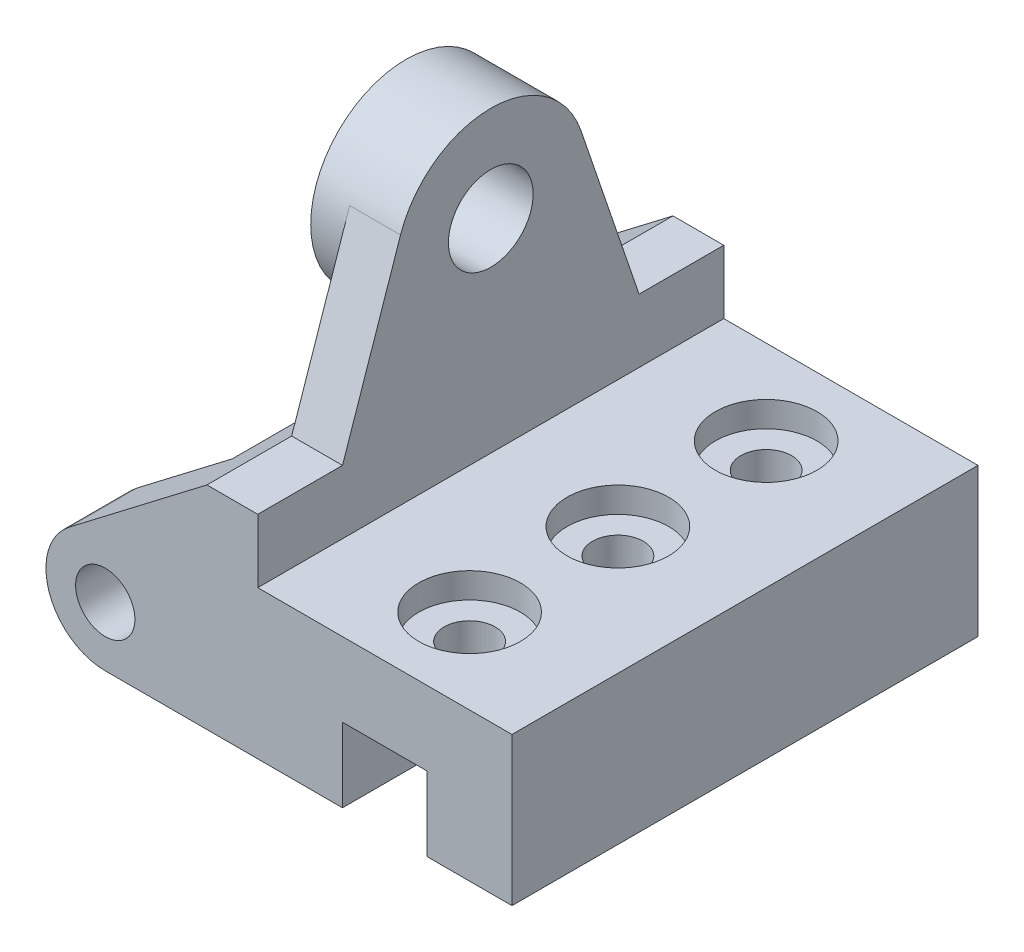
ISO-10303-21;
HEADER;
FILE_DESCRIPTION(('STEP AP214'),'2;1');
FILE_NAME('part.step','',(''),(''),'','','');
FILE_SCHEMA(('AUTOMOTIVE_DESIGN { 1 0 10303 214 1 1 1 1 }'));
ENDSEC;
DATA;
#1=APPLICATION_CONTEXT('core data for automotive mechanical design processes');
#2=APPLICATION_PROTOCOL_DEFINITION('international standard','automotive_design',2000,#1);
#3=PRODUCT_CONTEXT('',#1,'mechanical');
#4=PRODUCT('Part','Part','',(#3));
#5=PRODUCT_RELATED_PRODUCT_CATEGORY('part','',(#4));
#6=PRODUCT_DEFINITION_FORMATION('','',#4);
#7=PRODUCT_DEFINITION_CONTEXT('part definition',#1,'design');
#8=PRODUCT_DEFINITION('design','',#6,#7);
#9=PRODUCT_DEFINITION_SHAPE('','',#8);
#10=(LENGTH_UNIT() NAMED_UNIT(*) SI_UNIT(.MILLI.,.METRE.));
#11=(NAMED_UNIT(*) PLANE_ANGLE_UNIT() SI_UNIT($,.RADIAN.));
#12=(NAMED_UNIT(*) SI_UNIT($,.STERADIAN.) SOLID_ANGLE_UNIT());
#13=UNCERTAINTY_MEASURE_WITH_UNIT(LENGTH_MEASURE(1.E-05),#10,'distance_accuracy_value','');
#14=(GEOMETRIC_REPRESENTATION_CONTEXT(3) GLOBAL_UNCERTAINTY_ASSIGNED_CONTEXT((#13)) GLOBAL_UNIT_ASSIGNED_CONTEXT((#10,
#11,#12)) REPRESENTATION_CONTEXT('',''));
#15=CARTESIAN_POINT('',(0.,0.,0.));
#16=DIRECTION('',(0.,0.,1.));
#17=DIRECTION('',(1.,0.,0.));
#18=AXIS2_PLACEMENT_3D('',#15,#16,#17);
#19=CARTESIAN_POINT('',(24.,69.,0.));
#20=DIRECTION('',(1.,0.,0.));
#21=DIRECTION('',(0.,0.,-1.));
#22=AXIS2_PLACEMENT_3D('',#19,#20,#21);
#23=PLANE('',#22);
#24=CARTESIAN_POINT('',(24.,69.,0.));
#25=DIRECTION('',(-1.,0.,0.));
#26=DIRECTION('',(0.,0.,1.));
#27=AXIS2_PLACEMENT_3D('',#24,#25,#26);
#28=CIRCLE('',#27,22.5);
#29=CARTESIAN_POINT('',(24.,76.2499542674237,-21.2999568807138));
#30=VERTEX_POINT('',#29);
#31=CARTESIAN_POINT('',(24.,76.2499542674237,21.2999568807138));
#32=VERTEX_POINT('',#31);
#33=EDGE_CURVE('E176',#30,#32,#28,.T.);
#34=ORIENTED_EDGE('',*,*,#33,.F.);
#35=DIRECTION('',(0.,0.946664750253944,0.322220189663274));
#36=VECTOR('',#35,1.);
#37=CARTESIAN_POINT('',(24.,36.,-35.));
#38=LINE('',#37,#36);
#39=CARTESIAN_POINT('',(24.,36.,-35.));
#40=VERTEX_POINT('',#39);
#41=EDGE_CURVE('E189',#40,#30,#38,.T.);
#42=ORIENTED_EDGE('',*,*,#41,.F.);
#43=DIRECTION('',(0.,0.,-1.));
#44=VECTOR('',#43,1.);
#45=CARTESIAN_POINT('',(24.,36.,-35.));
#46=LINE('',#45,#44);
#47=CARTESIAN_POINT('',(24.,36.,35.));
#48=VERTEX_POINT('',#47);
#49=EDGE_CURVE('E181',#48,#40,#46,.T.);
#50=ORIENTED_EDGE('',*,*,#49,.F.);
#51=DIRECTION('',(0.,-0.946664750253944,0.322220189663275));
#52=VECTOR('',#51,1.);
#53=CARTESIAN_POINT('',(24.,76.2499542674237,21.2999568807137));
#54=LINE('',#53,#52);
#55=EDGE_CURVE('E178',#32,#48,#54,.T.);
#56=ORIENTED_EDGE('',*,*,#55,.F.);
#57=EDGE_LOOP('',(#34,#42,#50,#56));
#58=FACE_BOUND('',#57,.T.);
#59=ADVANCED_FACE('F43',(#58),#23,.F.);
#60=CARTESIAN_POINT('',(36.,36.,-55.));
#61=DIRECTION('',(0.,1.,0.));
#62=DIRECTION('',(-1.,0.,0.));
#63=AXIS2_PLACEMENT_3D('',#60,#61,#62);
#64=PLANE('',#63);
#65=DIRECTION('',(0.,0.,1.));
#66=VECTOR('',#65,1.);
#67=CARTESIAN_POINT('',(24.,36.,-55.));
#68=LINE('',#67,#66);
#69=CARTESIAN_POINT('',(24.,36.,-55.));
#70=VERTEX_POINT('',#69);
#71=EDGE_CURVE('E317',#70,#40,#68,.T.);
#72=ORIENTED_EDGE('',*,*,#71,.T.);
#73=DIRECTION('',(1.,0.,0.));
#74=VECTOR('',#73,1.);
#75=CARTESIAN_POINT('',(24.,36.,-35.));
#76=LINE('',#75,#74);
#77=CARTESIAN_POINT('',(36.,36.,-35.));
#78=VERTEX_POINT('',#77);
#79=EDGE_CURVE('E188',#40,#78,#76,.T.);
#80=ORIENTED_EDGE('',*,*,#79,.T.);
#81=DIRECTION('',(0.,0.,1.));
#82=VECTOR('',#81,1.);
#83=CARTESIAN_POINT('',(36.,36.,-55.));
#84=LINE('',#83,#82);
#85=CARTESIAN_POINT('',(36.,36.,-55.));
#86=VERTEX_POINT('',#85);
#87=EDGE_CURVE('E323',#86,#78,#84,.T.);
#88=ORIENTED_EDGE('',*,*,#87,.F.);
#89=DIRECTION('',(-1.,0.,0.));
#90=VECTOR('',#89,1.);
#91=CARTESIAN_POINT('',(36.,36.,-55.));
#92=LINE('',#91,#90);
#93=EDGE_CURVE('E283',#86,#70,#92,.T.);
#94=ORIENTED_EDGE('',*,*,#93,.T.);
#95=EDGE_LOOP('',(#72,#80,#88,#94));
#96=FACE_BOUND('',#95,.T.);
#97=ADVANCED_FACE('F438',(#96),#64,.T.);
#98=CARTESIAN_POINT('',(0.,0.,-55.));
#99=DIRECTION('',(0.,0.,1.));
#100=DIRECTION('',(1.,0.,0.));
#101=AXIS2_PLACEMENT_3D('',#98,#99,#100);
#102=CYLINDRICAL_SURFACE('',#101,14.);
#103=CARTESIAN_POINT('',(0.,0.,39.));
#104=DIRECTION('',(0.,0.,1.));
#105=DIRECTION('',(1.,0.,0.));
#106=AXIS2_PLACEMENT_3D('',#103,#104,#105);
#107=CIRCLE('',#106,14.);
#108=CARTESIAN_POINT('',(0.,-14.,39.));
#109=VERTEX_POINT('',#108);
#110=CARTESIAN_POINT('',(-8.50921228973418,11.1172526376006,39.));
#111=VERTEX_POINT('',#110);
#112=EDGE_CURVE('E244',#109,#111,#107,.F.);
#113=ORIENTED_EDGE('',*,*,#112,.F.);
#114=DIRECTION('',(0.,0.,1.));
#115=VECTOR('',#114,1.);
#116=CARTESIAN_POINT('',(0.,-14.,-55.));
#117=LINE('',#116,#115);
#118=CARTESIAN_POINT('',(0.,-14.,55.));
#119=VERTEX_POINT('',#118);
#120=EDGE_CURVE('E289',#109,#119,#117,.T.);
#121=ORIENTED_EDGE('',*,*,#120,.T.);
#122=CARTESIAN_POINT('',(0.,0.,55.));
#123=DIRECTION('',(0.,0.,1.));
#124=DIRECTION('',(1.,0.,0.));
#125=AXIS2_PLACEMENT_3D('',#122,#123,#124);
#126=CIRCLE('',#125,14.);
#127=CARTESIAN_POINT('',(-8.50921228973418,11.1172526376006,55.));
#128=VERTEX_POINT('',#127);
#129=EDGE_CURVE('E246',#128,#119,#126,.T.);
#130=ORIENTED_EDGE('',*,*,#129,.F.);
#131=DIRECTION('',(0.,0.,1.));
#132=VECTOR('',#131,1.);
#133=CARTESIAN_POINT('',(-8.50921228973418,11.1172526376006,-55.));
#134=LINE('',#133,#132);
#135=EDGE_CURVE('E55',#111,#128,#134,.T.);
#136=ORIENTED_EDGE('',*,*,#135,.F.);
#137=EDGE_LOOP('',(#113,#121,#130,#136));
#138=FACE_BOUND('',#137,.T.);
#139=ADVANCED_FACE('F453',(#138),#102,.T.);
#140=CARTESIAN_POINT('',(0.,0.,-55.));
#141=DIRECTION('',(0.,0.,1.));
#142=DIRECTION('',(1.,0.,0.));
#143=AXIS2_PLACEMENT_3D('',#140,#141,#142);
#144=CYLINDRICAL_SURFACE('',#143,7.);
#145=CARTESIAN_POINT('',(0.,0.,39.));
#146=DIRECTION('',(0.,0.,1.));
#147=DIRECTION('',(1.,0.,0.));
#148=AXIS2_PLACEMENT_3D('',#145,#146,#147);
#149=CIRCLE('',#148,7.);
#150=CARTESIAN_POINT('',(7.,0.,39.));
#151=VERTEX_POINT('',#150);
#152=EDGE_CURVE('E239',#151,#151,#149,.F.);
#153=ORIENTED_EDGE('',*,*,#152,.T.);
#154=EDGE_LOOP('',(#153));
#155=FACE_BOUND('',#154,.T.);
#156=CARTESIAN_POINT('',(0.,0.,55.));
#157=DIRECTION('',(0.,0.,1.));
#158=DIRECTION('',(1.,0.,0.));
#159=AXIS2_PLACEMENT_3D('',#156,#157,#158);
#160=CIRCLE('',#159,7.);
#161=CARTESIAN_POINT('',(7.,0.,55.));
#162=VERTEX_POINT('',#161);
#163=EDGE_CURVE('E248',#162,#162,#160,.T.);
#164=ORIENTED_EDGE('',*,*,#163,.T.);
#165=EDGE_LOOP('',(#164));
#166=FACE_BOUND('',#165,.T.);
#167=ADVANCED_FACE('F466',(#155,#166),#144,.F.);
#168=CARTESIAN_POINT('',(0.,0.,-39.));
#169=DIRECTION('',(0.,0.,-1.));
#170=DIRECTION('',(-1.,0.,0.));
#171=AXIS2_PLACEMENT_3D('',#168,#169,#170);
#172=CIRCLE('',#171,14.);
#173=CARTESIAN_POINT('',(-8.50921228973418,11.1172526376006,-39.));
#174=VERTEX_POINT('',#173);
#175=CARTESIAN_POINT('',(0.,-14.,-39.));
#176=VERTEX_POINT('',#175);
#177=EDGE_CURVE('E67',#174,#176,#172,.F.);
#178=ORIENTED_EDGE('',*,*,#177,.F.);
#179=CARTESIAN_POINT('',(-8.50921228973418,11.1172526376006,-55.));
#180=VERTEX_POINT('',#179);
#181=EDGE_CURVE('E11',#180,#174,#134,.T.);
#182=ORIENTED_EDGE('',*,*,#181,.F.);
#183=CARTESIAN_POINT('',(0.,0.,-55.));
#184=DIRECTION('',(0.,0.,1.));
#185=DIRECTION('',(1.,0.,0.));
#186=AXIS2_PLACEMENT_3D('',#183,#184,#185);
#187=CIRCLE('',#186,14.);
#188=CARTESIAN_POINT('',(0.,-14.,-55.));
#189=VERTEX_POINT('',#188);
#190=EDGE_CURVE('E251',#180,#189,#187,.T.);
#191=ORIENTED_EDGE('',*,*,#190,.T.);
#192=EDGE_CURVE('E343',#189,#176,#117,.T.);
#193=ORIENTED_EDGE('',*,*,#192,.T.);
#194=EDGE_LOOP('',(#178,#182,#191,#193));
#195=FACE_BOUND('',#194,.T.);
#196=ADVANCED_FACE('F44',(#195),#102,.T.);
#197=CARTESIAN_POINT('',(24.,36.,-55.));
#198=DIRECTION('',(-0.607800877838156,0.794089474114326,0.));
#199=DIRECTION('',(-0.794089474114326,-0.607800877838156,0.));
#200=AXIS2_PLACEMENT_3D('',#197,#198,#199);
#201=PLANE('',#200);
#202=DIRECTION('',(0.794089474114326,0.607800877838156,0.));
#203=VECTOR('',#202,1.);
#204=CARTESIAN_POINT('',(24.,36.,39.));
#205=LINE('',#204,#203);
#206=CARTESIAN_POINT('',(14.,28.3459396245485,39.));
#207=VERTEX_POINT('',#206);
#208=EDGE_CURVE('E238',#111,#207,#205,.T.);
#209=ORIENTED_EDGE('',*,*,#208,.F.);
#210=ORIENTED_EDGE('',*,*,#135,.T.);
#211=DIRECTION('',(-0.794089474114326,-0.607800877838156,0.));
#212=VECTOR('',#211,1.);
#213=CARTESIAN_POINT('',(24.,36.,55.));
#214=LINE('',#213,#212);
#215=CARTESIAN_POINT('',(24.,36.,55.));
#216=VERTEX_POINT('',#215);
#217=EDGE_CURVE('E260',#216,#128,#214,.T.);
#218=ORIENTED_EDGE('',*,*,#217,.F.);
#219=EDGE_CURVE('E325',#48,#216,#68,.T.);
#220=ORIENTED_EDGE('',*,*,#219,.F.);
#221=ORIENTED_EDGE('',*,*,#49,.T.);
#222=ORIENTED_EDGE('',*,*,#71,.F.);
#223=DIRECTION('',(-0.794089474114326,-0.607800877838156,0.));
#224=VECTOR('',#223,1.);
#225=CARTESIAN_POINT('',(24.,36.,-55.));
#226=LINE('',#225,#224);
#227=EDGE_CURVE('E285',#70,#180,#226,.T.);
#228=ORIENTED_EDGE('',*,*,#227,.T.);
#229=ORIENTED_EDGE('',*,*,#181,.T.);
#230=DIRECTION('',(-0.794089474114326,-0.607800877838156,0.));
#231=VECTOR('',#230,1.);
#232=CARTESIAN_POINT('',(24.,36.,-39.));
#233=LINE('',#232,#231);
#234=CARTESIAN_POINT('',(14.,28.3459396245485,-39.));
#235=VERTEX_POINT('',#234);
#236=EDGE_CURVE('E237',#235,#174,#233,.T.);
#237=ORIENTED_EDGE('',*,*,#236,.F.);
#238=DIRECTION('',(0.,0.,-1.));
#239=VECTOR('',#238,1.);
#240=CARTESIAN_POINT('',(14.,28.3459396245485,-55.));
#241=LINE('',#240,#239);
#242=EDGE_CURVE('E245',#207,#235,#241,.T.);
#243=ORIENTED_EDGE('',*,*,#242,.F.);
#244=EDGE_LOOP('',(#209,#210,#218,#220,#221,#222,#228,#229,#237,#243));
#245=FACE_BOUND('',#244,.T.);
#246=ADVANCED_FACE('F434',(#245),#201,.T.);
#247=DIRECTION('',(1.,0.,0.));
#248=VECTOR('',#247,1.);
#249=CARTESIAN_POINT('',(24.,36.,35.));
#250=LINE('',#249,#248);
#251=CARTESIAN_POINT('',(36.,36.,35.));
#252=VERTEX_POINT('',#251);
#253=EDGE_CURVE('E197',#48,#252,#250,.T.);
#254=ORIENTED_EDGE('',*,*,#253,.F.);
#255=ORIENTED_EDGE('',*,*,#219,.T.);
#256=DIRECTION('',(-1.,0.,0.));
#257=VECTOR('',#256,1.);
#258=CARTESIAN_POINT('',(36.,36.,55.));
#259=LINE('',#258,#257);
#260=CARTESIAN_POINT('',(36.,36.,55.));
#261=VERTEX_POINT('',#260);
#262=EDGE_CURVE('E314',#261,#216,#259,.T.);
#263=ORIENTED_EDGE('',*,*,#262,.F.);
#264=EDGE_CURVE('E326',#252,#261,#84,.T.);
#265=ORIENTED_EDGE('',*,*,#264,.F.);
#266=EDGE_LOOP('',(#254,#255,#263,#265));
#267=FACE_BOUND('',#266,.T.);
#268=ADVANCED_FACE('F489',(#267),#64,.T.);
#269=CARTESIAN_POINT('',(36.,21.,-55.));
#270=DIRECTION('',(1.,0.,0.));
#271=DIRECTION('',(0.,0.,-1.));
#272=AXIS2_PLACEMENT_3D('',#269,#270,#271);
#273=PLANE('',#272);
#274=DIRECTION('',(0.,1.,0.));
#275=VECTOR('',#274,1.);
#276=CARTESIAN_POINT('',(36.,21.,55.));
#277=LINE('',#276,#275);
#278=CARTESIAN_POINT('',(36.,21.,55.));
#279=VERTEX_POINT('',#278);
#280=EDGE_CURVE('E313',#279,#261,#277,.T.);
#281=ORIENTED_EDGE('',*,*,#280,.F.);
#282=DIRECTION('',(0.,0.,1.));
#283=VECTOR('',#282,1.);
#284=CARTESIAN_POINT('',(36.,21.,-55.));
#285=LINE('',#284,#283);
#286=CARTESIAN_POINT('',(36.,21.,-55.));
#287=VERTEX_POINT('',#286);
#288=EDGE_CURVE('E330',#287,#279,#285,.T.);
#289=ORIENTED_EDGE('',*,*,#288,.F.);
#290=DIRECTION('',(0.,1.,0.));
#291=VECTOR('',#290,1.);
#292=CARTESIAN_POINT('',(36.,21.,-55.));
#293=LINE('',#292,#291);
#294=EDGE_CURVE('E279',#287,#86,#293,.T.);
#295=ORIENTED_EDGE('',*,*,#294,.T.);
#296=ORIENTED_EDGE('',*,*,#87,.T.);
#297=DIRECTION('',(0.,0.946664750253944,0.322220189663274));
#298=VECTOR('',#297,1.);
#299=CARTESIAN_POINT('',(36.,36.,-35.));
#300=LINE('',#299,#298);
#301=CARTESIAN_POINT('',(36.,76.2499542674237,-21.2999568807138));
#302=VERTEX_POINT('',#301);
#303=EDGE_CURVE('E58',#78,#302,#300,.T.);
#304=ORIENTED_EDGE('',*,*,#303,.T.);
#305=CARTESIAN_POINT('',(36.,69.,0.));
#306=DIRECTION('',(1.,0.,0.));
#307=DIRECTION('',(0.,0.,-1.));
#308=AXIS2_PLACEMENT_3D('',#305,#306,#307);
#309=CIRCLE('',#308,22.5);
#310=CARTESIAN_POINT('',(36.,76.2499542674237,21.2999568807137));
#311=VERTEX_POINT('',#310);
#312=EDGE_CURVE('E217',#302,#311,#309,.T.);
#313=ORIENTED_EDGE('',*,*,#312,.T.);
#314=DIRECTION('',(0.,-0.946664750253944,0.322220189663275));
#315=VECTOR('',#314,1.);
#316=CARTESIAN_POINT('',(36.,76.2499542674237,21.2999568807137));
#317=LINE('',#316,#315);
#318=EDGE_CURVE('E192',#311,#252,#317,.T.);
#319=ORIENTED_EDGE('',*,*,#318,.T.);
#320=ORIENTED_EDGE('',*,*,#264,.T.);
#321=EDGE_LOOP('',(#281,#289,#295,#296,#304,#313,#319,#320));
#322=FACE_BOUND('',#321,.T.);
#323=CARTESIAN_POINT('',(36.,69.,0.));
#324=DIRECTION('',(1.,0.,0.));
#325=DIRECTION('',(0.,0.,-1.));
#326=AXIS2_PLACEMENT_3D('',#323,#324,#325);
#327=CIRCLE('',#326,10.);
#328=CARTESIAN_POINT('',(36.,69.,-10.));
#329=VERTEX_POINT('',#328);
#330=EDGE_CURVE('E210',#329,#329,#327,.T.);
#331=ORIENTED_EDGE('',*,*,#330,.F.);
#332=EDGE_LOOP('',(#331));
#333=FACE_BOUND('',#332,.T.);
#334=ADVANCED_FACE('F392',(#322,#333),#273,.T.);
#335=CARTESIAN_POINT('',(96.,21.,-55.));
#336=DIRECTION('',(0.,1.,0.));
#337=DIRECTION('',(-1.,0.,0.));
#338=AXIS2_PLACEMENT_3D('',#335,#336,#337);
#339=PLANE('',#338);
#340=CARTESIAN_POINT('',(66.,21.,35.));
#341=DIRECTION('',(0.,1.,0.));
#342=DIRECTION('',(0.,0.,1.));
#343=AXIS2_PLACEMENT_3D('',#340,#341,#342);
#344=CIRCLE('',#343,12.);
#345=CARTESIAN_POINT('',(66.,21.,47.));
#346=VERTEX_POINT('',#345);
#347=EDGE_CURVE('E810',#346,#346,#344,.T.);
#348=ORIENTED_EDGE('',*,*,#347,.F.);
#349=EDGE_LOOP('',(#348));
#350=FACE_BOUND('',#349,.T.);
#351=CARTESIAN_POINT('',(66.,21.,0.));
#352=DIRECTION('',(0.,1.,0.));
#353=DIRECTION('',(0.,0.,1.));
#354=AXIS2_PLACEMENT_3D('',#351,#352,#353);
#355=CIRCLE('',#354,12.);
#356=CARTESIAN_POINT('',(66.,21.,12.));
#357=VERTEX_POINT('',#356);
#358=EDGE_CURVE('E364',#357,#357,#355,.T.);
#359=ORIENTED_EDGE('',*,*,#358,.F.);
#360=EDGE_LOOP('',(#359));
#361=FACE_BOUND('',#360,.T.);
#362=CARTESIAN_POINT('',(66.,21.,-35.));
#363=DIRECTION('',(0.,1.,0.));
#364=DIRECTION('',(0.,0.,1.));
#365=AXIS2_PLACEMENT_3D('',#362,#363,#364);
#366=CIRCLE('',#365,12.);
#367=CARTESIAN_POINT('',(66.,21.,-23.));
#368=VERTEX_POINT('',#367);
#369=EDGE_CURVE('E354',#368,#368,#366,.T.);
#370=ORIENTED_EDGE('',*,*,#369,.F.);
#371=EDGE_LOOP('',(#370));
#372=FACE_BOUND('',#371,.T.);
#373=DIRECTION('',(-1.,0.,0.));
#374=VECTOR('',#373,1.);
#375=CARTESIAN_POINT('',(96.,21.,55.));
#376=LINE('',#375,#374);
#377=CARTESIAN_POINT('',(96.,21.,55.));
#378=VERTEX_POINT('',#377);
#379=EDGE_CURVE('E306',#378,#279,#376,.T.);
#380=ORIENTED_EDGE('',*,*,#379,.F.);
#381=DIRECTION('',(0.,0.,1.));
#382=VECTOR('',#381,1.);
#383=CARTESIAN_POINT('',(96.,21.,-55.));
#384=LINE('',#383,#382);
#385=CARTESIAN_POINT('',(96.,21.,-55.));
#386=VERTEX_POINT('',#385);
#387=EDGE_CURVE('E328',#386,#378,#384,.T.);
#388=ORIENTED_EDGE('',*,*,#387,.F.);
#389=DIRECTION('',(-1.,0.,0.));
#390=VECTOR('',#389,1.);
#391=CARTESIAN_POINT('',(96.,21.,-55.));
#392=LINE('',#391,#390);
#393=EDGE_CURVE('E274',#386,#287,#392,.T.);
#394=ORIENTED_EDGE('',*,*,#393,.T.);
#395=ORIENTED_EDGE('',*,*,#288,.T.);
#396=EDGE_LOOP('',(#380,#388,#394,#395));
#397=FACE_BOUND('',#396,.T.);
#398=ADVANCED_FACE('F386',(#350,#361,#372,#397),#339,.T.);
#399=CARTESIAN_POINT('',(96.,-14.,-55.));
#400=DIRECTION('',(1.,0.,0.));
#401=DIRECTION('',(0.,0.,-1.));
#402=AXIS2_PLACEMENT_3D('',#399,#400,#401);
#403=PLANE('',#402);
#404=DIRECTION('',(0.,1.,0.));
#405=VECTOR('',#404,1.);
#406=CARTESIAN_POINT('',(96.,-14.,55.));
#407=LINE('',#406,#405);
#408=CARTESIAN_POINT('',(96.,-14.,55.));
#409=VERTEX_POINT('',#408);
#410=EDGE_CURVE('E301',#409,#378,#407,.T.);
#411=ORIENTED_EDGE('',*,*,#410,.F.);
#412=DIRECTION('',(0.,0.,1.));
#413=VECTOR('',#412,1.);
#414=CARTESIAN_POINT('',(96.,-14.,-55.));
#415=LINE('',#414,#413);
#416=CARTESIAN_POINT('',(96.,-14.,-55.));
#417=VERTEX_POINT('',#416);
#418=EDGE_CURVE('E332',#417,#409,#415,.T.);
#419=ORIENTED_EDGE('',*,*,#418,.F.);
#420=DIRECTION('',(0.,1.,0.));
#421=VECTOR('',#420,1.);
#422=CARTESIAN_POINT('',(96.,-14.,-55.));
#423=LINE('',#422,#421);
#424=EDGE_CURVE('E275',#417,#386,#423,.T.);
#425=ORIENTED_EDGE('',*,*,#424,.T.);
#426=ORIENTED_EDGE('',*,*,#387,.T.);
#427=EDGE_LOOP('',(#411,#419,#425,#426));
#428=FACE_BOUND('',#427,.T.);
#429=ADVANCED_FACE('F394',(#428),#403,.T.);
#430=CARTESIAN_POINT('',(76.,-14.,-55.));
#431=DIRECTION('',(0.,-1.,0.));
#432=DIRECTION('',(0.,0.,-1.));
#433=AXIS2_PLACEMENT_3D('',#430,#431,#432);
#434=PLANE('',#433);
#435=DIRECTION('',(1.,0.,0.));
#436=VECTOR('',#435,1.);
#437=CARTESIAN_POINT('',(76.,-14.,55.));
#438=LINE('',#437,#436);
#439=CARTESIAN_POINT('',(76.,-14.,55.));
#440=VERTEX_POINT('',#439);
#441=EDGE_CURVE('E304',#440,#409,#438,.T.);
#442=ORIENTED_EDGE('',*,*,#441,.F.);
#443=DIRECTION('',(0.,0.,1.));
#444=VECTOR('',#443,1.);
#445=CARTESIAN_POINT('',(76.,-14.,-55.));
#446=LINE('',#445,#444);
#447=CARTESIAN_POINT('',(76.,-14.,-55.));
#448=VERTEX_POINT('',#447);
#449=EDGE_CURVE('E334',#448,#440,#446,.T.);
#450=ORIENTED_EDGE('',*,*,#449,.F.);
#451=DIRECTION('',(1.,0.,0.));
#452=VECTOR('',#451,1.);
#453=CARTESIAN_POINT('',(76.,-14.,-55.));
#454=LINE('',#453,#452);
#455=EDGE_CURVE('E267',#448,#417,#454,.T.);
#456=ORIENTED_EDGE('',*,*,#455,.T.);
#457=ORIENTED_EDGE('',*,*,#418,.T.);
#458=EDGE_LOOP('',(#442,#450,#456,#457));
#459=FACE_BOUND('',#458,.T.);
#460=ADVANCED_FACE('F414',(#459),#434,.T.);
#461=CARTESIAN_POINT('',(76.,3.5,-55.));
#462=DIRECTION('',(-1.,0.,0.));
#463=DIRECTION('',(0.,0.,1.));
#464=AXIS2_PLACEMENT_3D('',#461,#462,#463);
#465=PLANE('',#464);
#466=DIRECTION('',(0.,-1.,0.));
#467=VECTOR('',#466,1.);
#468=CARTESIAN_POINT('',(76.,3.5,55.));
#469=LINE('',#468,#467);
#470=CARTESIAN_POINT('',(76.,3.5,55.));
#471=VERTEX_POINT('',#470);
#472=EDGE_CURVE('E300',#471,#440,#469,.T.);
#473=ORIENTED_EDGE('',*,*,#472,.F.);
#474=DIRECTION('',(0.,0.,1.));
#475=VECTOR('',#474,1.);
#476=CARTESIAN_POINT('',(76.,3.5,-55.));
#477=LINE('',#476,#475);
#478=CARTESIAN_POINT('',(76.,3.5,-55.));
#479=VERTEX_POINT('',#478);
#480=EDGE_CURVE('E333',#479,#471,#477,.T.);
#481=ORIENTED_EDGE('',*,*,#480,.F.);
#482=DIRECTION('',(0.,-1.,0.));
#483=VECTOR('',#482,1.);
#484=CARTESIAN_POINT('',(76.,3.5,-55.));
#485=LINE('',#484,#483);
#486=EDGE_CURVE('E266',#479,#448,#485,.T.);
#487=ORIENTED_EDGE('',*,*,#486,.T.);
#488=ORIENTED_EDGE('',*,*,#449,.T.);
#489=EDGE_LOOP('',(#473,#481,#487,#488));
#490=FACE_BOUND('',#489,.T.);
#491=ADVANCED_FACE('F411',(#490),#465,.T.);
#492=CARTESIAN_POINT('',(56.,3.5,-55.));
#493=DIRECTION('',(0.,-1.,0.));
#494=DIRECTION('',(0.,0.,-1.));
#495=AXIS2_PLACEMENT_3D('',#492,#493,#494);
#496=PLANE('',#495);
#497=CARTESIAN_POINT('',(66.,3.5,35.));
#498=DIRECTION('',(0.,-1.,0.));
#499=DIRECTION('',(0.,0.,-1.));
#500=AXIS2_PLACEMENT_3D('',#497,#498,#499);
#501=CIRCLE('',#500,6.00000000000001);
#502=CARTESIAN_POINT('',(66.,3.5,29.));
#503=VERTEX_POINT('',#502);
#504=EDGE_CURVE('E50',#503,#503,#501,.T.);
#505=ORIENTED_EDGE('',*,*,#504,.F.);
#506=EDGE_LOOP('',(#505));
#507=FACE_BOUND('',#506,.T.);
#508=CARTESIAN_POINT('',(66.,3.5,0.));
#509=DIRECTION('',(0.,-1.,0.));
#510=DIRECTION('',(0.,0.,-1.));
#511=AXIS2_PLACEMENT_3D('',#508,#509,#510);
#512=CIRCLE('',#511,6.00000000000001);
#513=CARTESIAN_POINT('',(66.,3.5,-6.00000000000001));
#514=VERTEX_POINT('',#513);
#515=EDGE_CURVE('E348',#514,#514,#512,.T.);
#516=ORIENTED_EDGE('',*,*,#515,.F.);
#517=EDGE_LOOP('',(#516));
#518=FACE_BOUND('',#517,.T.);
#519=CARTESIAN_POINT('',(66.,3.5,-35.));
#520=DIRECTION('',(0.,-1.,0.));
#521=DIRECTION('',(0.,0.,-1.));
#522=AXIS2_PLACEMENT_3D('',#519,#520,#521);
#523=CIRCLE('',#522,6.00000000000001);
#524=CARTESIAN_POINT('',(66.,3.5,-41.));
#525=VERTEX_POINT('',#524);
#526=EDGE_CURVE('E209',#525,#525,#523,.T.);
#527=ORIENTED_EDGE('',*,*,#526,.F.);
#528=EDGE_LOOP('',(#527));
#529=FACE_BOUND('',#528,.T.);
#530=DIRECTION('',(1.,0.,0.));
#531=VECTOR('',#530,1.);
#532=CARTESIAN_POINT('',(56.,3.5,55.));
#533=LINE('',#532,#531);
#534=CARTESIAN_POINT('',(56.,3.5,55.));
#535=VERTEX_POINT('',#534);
#536=EDGE_CURVE('E298',#535,#471,#533,.T.);
#537=ORIENTED_EDGE('',*,*,#536,.F.);
#538=DIRECTION('',(0.,0.,1.));
#539=VECTOR('',#538,1.);
#540=CARTESIAN_POINT('',(56.,3.5,-55.));
#541=LINE('',#540,#539);
#542=CARTESIAN_POINT('',(56.,3.5,-55.));
#543=VERTEX_POINT('',#542);
#544=EDGE_CURVE('E339',#543,#535,#541,.T.);
#545=ORIENTED_EDGE('',*,*,#544,.F.);
#546=DIRECTION('',(1.,0.,0.));
#547=VECTOR('',#546,1.);
#548=CARTESIAN_POINT('',(56.,3.5,-55.));
#549=LINE('',#548,#547);
#550=EDGE_CURVE('E263',#543,#479,#549,.T.);
#551=ORIENTED_EDGE('',*,*,#550,.T.);
#552=ORIENTED_EDGE('',*,*,#480,.T.);
#553=EDGE_LOOP('',(#537,#545,#551,#552));
#554=FACE_BOUND('',#553,.T.);
#555=ADVANCED_FACE('F419',(#507,#518,#529,#554),#496,.T.);
#556=CARTESIAN_POINT('',(56.,-14.,-55.));
#557=DIRECTION('',(1.,0.,0.));
#558=DIRECTION('',(0.,0.,-1.));
#559=AXIS2_PLACEMENT_3D('',#556,#557,#558);
#560=PLANE('',#559);
#561=DIRECTION('',(0.,1.,0.));
#562=VECTOR('',#561,1.);
#563=CARTESIAN_POINT('',(56.,-14.,55.));
#564=LINE('',#563,#562);
#565=CARTESIAN_POINT('',(56.,-14.,55.));
#566=VERTEX_POINT('',#565);
#567=EDGE_CURVE('E291',#566,#535,#564,.T.);
#568=ORIENTED_EDGE('',*,*,#567,.F.);
#569=DIRECTION('',(0.,0.,1.));
#570=VECTOR('',#569,1.);
#571=CARTESIAN_POINT('',(56.,-14.,-55.));
#572=LINE('',#571,#570);
#573=CARTESIAN_POINT('',(56.,-14.,-55.));
#574=VERTEX_POINT('',#573);
#575=EDGE_CURVE('E340',#574,#566,#572,.T.);
#576=ORIENTED_EDGE('',*,*,#575,.F.);
#577=DIRECTION('',(0.,1.,0.));
#578=VECTOR('',#577,1.);
#579=CARTESIAN_POINT('',(56.,-14.,-55.));
#580=LINE('',#579,#578);
#581=EDGE_CURVE('E257',#574,#543,#580,.T.);
#582=ORIENTED_EDGE('',*,*,#581,.T.);
#583=ORIENTED_EDGE('',*,*,#544,.T.);
#584=EDGE_LOOP('',(#568,#576,#582,#583));
#585=FACE_BOUND('',#584,.T.);
#586=ADVANCED_FACE('F421',(#585),#560,.T.);
#587=CARTESIAN_POINT('',(0.,-14.,-55.));
#588=DIRECTION('',(0.,-1.,0.));
#589=DIRECTION('',(0.,0.,-1.));
#590=AXIS2_PLACEMENT_3D('',#587,#588,#589);
#591=PLANE('',#590);
#592=DIRECTION('',(-1.,0.,0.));
#593=VECTOR('',#592,1.);
#594=CARTESIAN_POINT('',(-14.,-14.,39.));
#595=LINE('',#594,#593);
#596=CARTESIAN_POINT('',(14.,-14.,39.));
#597=VERTEX_POINT('',#596);
#598=EDGE_CURVE('E230',#597,#109,#595,.T.);
#599=ORIENTED_EDGE('',*,*,#598,.F.);
#600=DIRECTION('',(0.,0.,1.));
#601=VECTOR('',#600,1.);
#602=CARTESIAN_POINT('',(14.,-14.,39.));
#603=LINE('',#602,#601);
#604=CARTESIAN_POINT('',(14.,-14.,-39.));
#605=VERTEX_POINT('',#604);
#606=EDGE_CURVE('E228',#605,#597,#603,.T.);
#607=ORIENTED_EDGE('',*,*,#606,.F.);
#608=DIRECTION('',(1.,0.,0.));
#609=VECTOR('',#608,1.);
#610=CARTESIAN_POINT('',(-14.,-14.,-39.));
#611=LINE('',#610,#609);
#612=EDGE_CURVE('E222',#176,#605,#611,.T.);
#613=ORIENTED_EDGE('',*,*,#612,.F.);
#614=ORIENTED_EDGE('',*,*,#192,.F.);
#615=DIRECTION('',(1.,0.,0.));
#616=VECTOR('',#615,1.);
#617=CARTESIAN_POINT('',(0.,-14.,-55.));
#618=LINE('',#617,#616);
#619=EDGE_CURVE('E258',#189,#574,#618,.T.);
#620=ORIENTED_EDGE('',*,*,#619,.T.);
#621=ORIENTED_EDGE('',*,*,#575,.T.);
#622=DIRECTION('',(1.,0.,0.));
#623=VECTOR('',#622,1.);
#624=CARTESIAN_POINT('',(0.,-14.,55.));
#625=LINE('',#624,#623);
#626=EDGE_CURVE('E286',#119,#566,#625,.T.);
#627=ORIENTED_EDGE('',*,*,#626,.F.);
#628=ORIENTED_EDGE('',*,*,#120,.F.);
#629=EDGE_LOOP('',(#599,#607,#613,#614,#620,#621,#627,#628));
#630=FACE_BOUND('',#629,.T.);
#631=ADVANCED_FACE('F430',(#630),#591,.T.);
#632=CARTESIAN_POINT('',(0.,0.,-55.));
#633=DIRECTION('',(0.,0.,1.));
#634=DIRECTION('',(1.,0.,0.));
#635=AXIS2_PLACEMENT_3D('',#632,#633,#634);
#636=PLANE('',#635);
#637=CARTESIAN_POINT('',(0.,0.,-55.));
#638=DIRECTION('',(0.,0.,1.));
#639=DIRECTION('',(1.,0.,0.));
#640=AXIS2_PLACEMENT_3D('',#637,#638,#639);
#641=CIRCLE('',#640,7.);
#642=CARTESIAN_POINT('',(7.,0.,-55.));
#643=VERTEX_POINT('',#642);
#644=EDGE_CURVE('E249',#643,#643,#641,.T.);
#645=ORIENTED_EDGE('',*,*,#644,.T.);
#646=EDGE_LOOP('',(#645));
#647=FACE_BOUND('',#646,.T.);
#648=ORIENTED_EDGE('',*,*,#190,.F.);
#649=ORIENTED_EDGE('',*,*,#227,.F.);
#650=ORIENTED_EDGE('',*,*,#93,.F.);
#651=ORIENTED_EDGE('',*,*,#294,.F.);
#652=ORIENTED_EDGE('',*,*,#393,.F.);
#653=ORIENTED_EDGE('',*,*,#424,.F.);
#654=ORIENTED_EDGE('',*,*,#455,.F.);
#655=ORIENTED_EDGE('',*,*,#486,.F.);
#656=ORIENTED_EDGE('',*,*,#550,.F.);
#657=ORIENTED_EDGE('',*,*,#581,.F.);
#658=ORIENTED_EDGE('',*,*,#619,.F.);
#659=EDGE_LOOP('',(#648,#649,#650,#651,#652,#653,#654,#655,#656,#657,#658));
#660=FACE_BOUND('',#659,.T.);
#661=ADVANCED_FACE('F407',(#647,#660),#636,.F.);
#662=CARTESIAN_POINT('',(0.,0.,55.));
#663=DIRECTION('',(0.,0.,1.));
#664=DIRECTION('',(1.,0.,0.));
#665=AXIS2_PLACEMENT_3D('',#662,#663,#664);
#666=PLANE('',#665);
#667=ORIENTED_EDGE('',*,*,#163,.F.);
#668=EDGE_LOOP('',(#667));
#669=FACE_BOUND('',#668,.T.);
#670=ORIENTED_EDGE('',*,*,#129,.T.);
#671=ORIENTED_EDGE('',*,*,#626,.T.);
#672=ORIENTED_EDGE('',*,*,#567,.T.);
#673=ORIENTED_EDGE('',*,*,#536,.T.);
#674=ORIENTED_EDGE('',*,*,#472,.T.);
#675=ORIENTED_EDGE('',*,*,#441,.T.);
#676=ORIENTED_EDGE('',*,*,#410,.T.);
#677=ORIENTED_EDGE('',*,*,#379,.T.);
#678=ORIENTED_EDGE('',*,*,#280,.T.);
#679=ORIENTED_EDGE('',*,*,#262,.T.);
#680=ORIENTED_EDGE('',*,*,#217,.T.);
#681=EDGE_LOOP('',(#670,#671,#672,#673,#674,#675,#676,#677,#678,#679,#680));
#682=FACE_BOUND('',#681,.T.);
#683=ADVANCED_FACE('F402',(#669,#682),#666,.T.);
#684=CARTESIAN_POINT('',(0.,0.,-39.));
#685=DIRECTION('',(0.,0.,-1.));
#686=DIRECTION('',(-1.,0.,0.));
#687=AXIS2_PLACEMENT_3D('',#684,#685,#686);
#688=CIRCLE('',#687,7.);
#689=CARTESIAN_POINT('',(-7.,0.,-39.));
#690=VERTEX_POINT('',#689);
#691=EDGE_CURVE('E235',#690,#690,#688,.F.);
#692=ORIENTED_EDGE('',*,*,#691,.T.);
#693=EDGE_LOOP('',(#692));
#694=FACE_BOUND('',#693,.T.);
#695=ORIENTED_EDGE('',*,*,#644,.F.);
#696=EDGE_LOOP('',(#695));
#697=FACE_BOUND('',#696,.T.);
#698=ADVANCED_FACE('F468',(#694,#697),#144,.F.);
#699=CARTESIAN_POINT('',(-14.,96.,39.));
#700=DIRECTION('',(0.,0.,1.));
#701=DIRECTION('',(1.,0.,0.));
#702=AXIS2_PLACEMENT_3D('',#699,#700,#701);
#703=PLANE('',#702);
#704=ORIENTED_EDGE('',*,*,#112,.T.);
#705=ORIENTED_EDGE('',*,*,#208,.T.);
#706=DIRECTION('',(0.,-1.,0.));
#707=VECTOR('',#706,1.);
#708=CARTESIAN_POINT('',(14.,96.,39.));
#709=LINE('',#708,#707);
#710=EDGE_CURVE('E234',#207,#597,#709,.T.);
#711=ORIENTED_EDGE('',*,*,#710,.T.);
#712=ORIENTED_EDGE('',*,*,#598,.T.);
#713=EDGE_LOOP('',(#704,#705,#711,#712));
#714=FACE_BOUND('',#713,.T.);
#715=ORIENTED_EDGE('',*,*,#152,.F.);
#716=EDGE_LOOP('',(#715));
#717=FACE_BOUND('',#716,.T.);
#718=ADVANCED_FACE('F455',(#714,#717),#703,.F.);
#719=CARTESIAN_POINT('',(-14.,96.,-39.));
#720=DIRECTION('',(0.,0.,-1.));
#721=DIRECTION('',(-1.,0.,0.));
#722=AXIS2_PLACEMENT_3D('',#719,#720,#721);
#723=PLANE('',#722);
#724=ORIENTED_EDGE('',*,*,#177,.T.);
#725=ORIENTED_EDGE('',*,*,#612,.T.);
#726=DIRECTION('',(0.,-1.,0.));
#727=VECTOR('',#726,1.);
#728=CARTESIAN_POINT('',(14.,96.,-39.));
#729=LINE('',#728,#727);
#730=EDGE_CURVE('E233',#235,#605,#729,.T.);
#731=ORIENTED_EDGE('',*,*,#730,.F.);
#732=ORIENTED_EDGE('',*,*,#236,.T.);
#733=EDGE_LOOP('',(#724,#725,#731,#732));
#734=FACE_BOUND('',#733,.T.);
#735=ORIENTED_EDGE('',*,*,#691,.F.);
#736=EDGE_LOOP('',(#735));
#737=FACE_BOUND('',#736,.T.);
#738=ADVANCED_FACE('F458',(#734,#737),#723,.F.);
#739=CARTESIAN_POINT('',(14.,96.,39.));
#740=DIRECTION('',(1.,0.,0.));
#741=DIRECTION('',(0.,0.,-1.));
#742=AXIS2_PLACEMENT_3D('',#739,#740,#741);
#743=PLANE('',#742);
#744=ORIENTED_EDGE('',*,*,#242,.T.);
#745=ORIENTED_EDGE('',*,*,#730,.T.);
#746=ORIENTED_EDGE('',*,*,#606,.T.);
#747=ORIENTED_EDGE('',*,*,#710,.F.);
#748=EDGE_LOOP('',(#744,#745,#746,#747));
#749=FACE_BOUND('',#748,.T.);
#750=ADVANCED_FACE('F456',(#749),#743,.F.);
#751=CARTESIAN_POINT('',(24.,76.2499542674237,21.2999568807137));
#752=DIRECTION('',(0.,0.322220189663275,0.946664750253944));
#753=DIRECTION('',(0.,-0.946664750253945,0.322220189663275));
#754=AXIS2_PLACEMENT_3D('',#751,#752,#753);
#755=PLANE('',#754);
#756=ORIENTED_EDGE('',*,*,#318,.F.);
#757=DIRECTION('',(1.,0.,0.));
#758=VECTOR('',#757,1.);
#759=CARTESIAN_POINT('',(24.,76.2499542674237,21.2999568807137));
#760=LINE('',#759,#758);
#761=EDGE_CURVE('E186',#32,#311,#760,.T.);
#762=ORIENTED_EDGE('',*,*,#761,.F.);
#763=ORIENTED_EDGE('',*,*,#55,.T.);
#764=ORIENTED_EDGE('',*,*,#253,.T.);
#765=EDGE_LOOP('',(#756,#762,#763,#764));
#766=FACE_BOUND('',#765,.T.);
#767=ADVANCED_FACE('F193',(#766),#755,.T.);
#768=CARTESIAN_POINT('',(24.,69.,0.));
#769=DIRECTION('',(1.,0.,0.));
#770=DIRECTION('',(0.,0.,-1.));
#771=AXIS2_PLACEMENT_3D('',#768,#769,#770);
#772=CYLINDRICAL_SURFACE('',#771,22.5);
#773=ORIENTED_EDGE('',*,*,#312,.F.);
#774=DIRECTION('',(1.,0.,0.));
#775=VECTOR('',#774,1.);
#776=CARTESIAN_POINT('',(24.,76.2499542674237,-21.2999568807138));
#777=LINE('',#776,#775);
#778=EDGE_CURVE('E196',#30,#302,#777,.T.);
#779=ORIENTED_EDGE('',*,*,#778,.F.);
#780=ORIENTED_EDGE('',*,*,#33,.T.);
#781=ORIENTED_EDGE('',*,*,#761,.T.);
#782=EDGE_LOOP('',(#773,#779,#780,#781));
#783=FACE_BOUND('',#782,.T.);
#784=CARTESIAN_POINT('',(16.,69.,0.));
#785=DIRECTION('',(-1.,0.,0.));
#786=DIRECTION('',(0.,0.,1.));
#787=AXIS2_PLACEMENT_3D('',#784,#785,#786);
#788=CIRCLE('',#787,22.5);
#789=CARTESIAN_POINT('',(16.,69.,22.5));
#790=VERTEX_POINT('',#789);
#791=EDGE_CURVE('E201',#790,#790,#788,.T.);
#792=ORIENTED_EDGE('',*,*,#791,.F.);
#793=EDGE_LOOP('',(#792));
#794=FACE_BOUND('',#793,.T.);
#795=ADVANCED_FACE('F199',(#783,#794),#772,.T.);
#796=CARTESIAN_POINT('',(24.,36.,-35.));
#797=DIRECTION('',(0.,0.322220189663275,-0.946664750253945));
#798=DIRECTION('',(0.,0.946664750253945,0.322220189663275));
#799=AXIS2_PLACEMENT_3D('',#796,#797,#798);
#800=PLANE('',#799);
#801=ORIENTED_EDGE('',*,*,#303,.F.);
#802=ORIENTED_EDGE('',*,*,#79,.F.);
#803=ORIENTED_EDGE('',*,*,#41,.T.);
#804=ORIENTED_EDGE('',*,*,#778,.T.);
#805=EDGE_LOOP('',(#801,#802,#803,#804));
#806=FACE_BOUND('',#805,.T.);
#807=ADVANCED_FACE('F500',(#806),#800,.T.);
#808=CARTESIAN_POINT('',(24.,69.,0.));
#809=DIRECTION('',(1.,0.,0.));
#810=DIRECTION('',(0.,0.,-1.));
#811=AXIS2_PLACEMENT_3D('',#808,#809,#810);
#812=CYLINDRICAL_SURFACE('',#811,10.);
#813=ORIENTED_EDGE('',*,*,#330,.T.);
#814=EDGE_LOOP('',(#813));
#815=FACE_BOUND('',#814,.T.);
#816=CARTESIAN_POINT('',(16.,69.,0.));
#817=DIRECTION('',(-1.,0.,0.));
#818=DIRECTION('',(0.,0.,1.));
#819=AXIS2_PLACEMENT_3D('',#816,#817,#818);
#820=CIRCLE('',#819,10.);
#821=CARTESIAN_POINT('',(16.,69.,10.));
#822=VERTEX_POINT('',#821);
#823=EDGE_CURVE('E204',#822,#822,#820,.T.);
#824=ORIENTED_EDGE('',*,*,#823,.T.);
#825=EDGE_LOOP('',(#824));
#826=FACE_BOUND('',#825,.T.);
#827=ADVANCED_FACE('F492',(#815,#826),#812,.F.);
#828=CARTESIAN_POINT('',(16.,69.,0.));
#829=DIRECTION('',(-1.,0.,0.));
#830=DIRECTION('',(0.,0.,1.));
#831=AXIS2_PLACEMENT_3D('',#828,#829,#830);
#832=PLANE('',#831);
#833=ORIENTED_EDGE('',*,*,#791,.T.);
#834=EDGE_LOOP('',(#833));
#835=FACE_BOUND('',#834,.T.);
#836=ORIENTED_EDGE('',*,*,#823,.F.);
#837=EDGE_LOOP('',(#836));
#838=FACE_BOUND('',#837,.T.);
#839=ADVANCED_FACE('F564',(#835,#838),#832,.T.);
#840=CARTESIAN_POINT('',(66.,21.,-35.));
#841=DIRECTION('',(0.,1.,0.));
#842=DIRECTION('',(0.,0.,1.));
#843=AXIS2_PLACEMENT_3D('',#840,#841,#842);
#844=CYLINDRICAL_SURFACE('',#843,6.00000000000001);
#845=ORIENTED_EDGE('',*,*,#526,.T.);
#846=EDGE_LOOP('',(#845));
#847=FACE_BOUND('',#846,.T.);
#848=CARTESIAN_POINT('',(66.,15.,-35.));
#849=DIRECTION('',(0.,1.,0.));
#850=DIRECTION('',(0.,0.,1.));
#851=AXIS2_PLACEMENT_3D('',#848,#849,#850);
#852=CIRCLE('',#851,6.00000000000002);
#853=CARTESIAN_POINT('',(66.,15.,-29.));
#854=VERTEX_POINT('',#853);
#855=EDGE_CURVE('E349',#854,#854,#852,.T.);
#856=ORIENTED_EDGE('',*,*,#855,.T.);
#857=EDGE_LOOP('',(#856));
#858=FACE_BOUND('',#857,.T.);
#859=ADVANCED_FACE('F372',(#847,#858),#844,.F.);
#860=CARTESIAN_POINT('',(72.,15.,-35.));
#861=DIRECTION('',(0.,-1.,0.));
#862=DIRECTION('',(0.,0.,-1.));
#863=AXIS2_PLACEMENT_3D('',#860,#861,#862);
#864=PLANE('',#863);
#865=ORIENTED_EDGE('',*,*,#855,.F.);
#866=EDGE_LOOP('',(#865));
#867=FACE_BOUND('',#866,.T.);
#868=CARTESIAN_POINT('',(66.,15.,-35.));
#869=DIRECTION('',(0.,1.,0.));
#870=DIRECTION('',(0.,0.,1.));
#871=AXIS2_PLACEMENT_3D('',#868,#869,#870);
#872=CIRCLE('',#871,12.);
#873=CARTESIAN_POINT('',(66.,15.,-23.));
#874=VERTEX_POINT('',#873);
#875=EDGE_CURVE('E359',#874,#874,#872,.T.);
#876=ORIENTED_EDGE('',*,*,#875,.T.);
#877=EDGE_LOOP('',(#876));
#878=FACE_BOUND('',#877,.T.);
#879=ADVANCED_FACE('F376',(#867,#878),#864,.F.);
#880=CARTESIAN_POINT('',(66.,21.,-35.));
#881=DIRECTION('',(0.,1.,0.));
#882=DIRECTION('',(0.,0.,1.));
#883=AXIS2_PLACEMENT_3D('',#880,#881,#882);
#884=CYLINDRICAL_SURFACE('',#883,12.);
#885=ORIENTED_EDGE('',*,*,#875,.F.);
#886=EDGE_LOOP('',(#885));
#887=FACE_BOUND('',#886,.T.);
#888=ORIENTED_EDGE('',*,*,#369,.T.);
#889=EDGE_LOOP('',(#888));
#890=FACE_BOUND('',#889,.T.);
#891=ADVANCED_FACE('F377',(#887,#890),#884,.F.);
#892=CARTESIAN_POINT('',(66.,21.,0.));
#893=DIRECTION('',(0.,1.,0.));
#894=DIRECTION('',(0.,0.,1.));
#895=AXIS2_PLACEMENT_3D('',#892,#893,#894);
#896=CYLINDRICAL_SURFACE('',#895,6.00000000000001);
#897=ORIENTED_EDGE('',*,*,#515,.T.);
#898=EDGE_LOOP('',(#897));
#899=FACE_BOUND('',#898,.T.);
#900=CARTESIAN_POINT('',(66.,15.,0.));
#901=DIRECTION('',(0.,1.,0.));
#902=DIRECTION('',(0.,0.,1.));
#903=AXIS2_PLACEMENT_3D('',#900,#901,#902);
#904=CIRCLE('',#903,6.00000000000002);
#905=CARTESIAN_POINT('',(66.,15.,6.00000000000002));
#906=VERTEX_POINT('',#905);
#907=EDGE_CURVE('E352',#906,#906,#904,.T.);
#908=ORIENTED_EDGE('',*,*,#907,.T.);
#909=EDGE_LOOP('',(#908));
#910=FACE_BOUND('',#909,.T.);
#911=ADVANCED_FACE('F384',(#899,#910),#896,.F.);
#912=CARTESIAN_POINT('',(72.,15.,0.));
#913=DIRECTION('',(0.,-1.,0.));
#914=DIRECTION('',(0.,0.,-1.));
#915=AXIS2_PLACEMENT_3D('',#912,#913,#914);
#916=PLANE('',#915);
#917=ORIENTED_EDGE('',*,*,#907,.F.);
#918=EDGE_LOOP('',(#917));
#919=FACE_BOUND('',#918,.T.);
#920=CARTESIAN_POINT('',(66.,15.,0.));
#921=DIRECTION('',(0.,1.,0.));
#922=DIRECTION('',(0.,0.,1.));
#923=AXIS2_PLACEMENT_3D('',#920,#921,#922);
#924=CIRCLE('',#923,12.);
#925=CARTESIAN_POINT('',(66.,15.,12.));
#926=VERTEX_POINT('',#925);
#927=EDGE_CURVE('E356',#926,#926,#924,.T.);
#928=ORIENTED_EDGE('',*,*,#927,.T.);
#929=EDGE_LOOP('',(#928));
#930=FACE_BOUND('',#929,.T.);
#931=ADVANCED_FACE('F602',(#919,#930),#916,.F.);
#932=CARTESIAN_POINT('',(66.,21.,0.));
#933=DIRECTION('',(0.,1.,0.));
#934=DIRECTION('',(0.,0.,1.));
#935=AXIS2_PLACEMENT_3D('',#932,#933,#934);
#936=CYLINDRICAL_SURFACE('',#935,12.);
#937=ORIENTED_EDGE('',*,*,#927,.F.);
#938=EDGE_LOOP('',(#937));
#939=FACE_BOUND('',#938,.T.);
#940=ORIENTED_EDGE('',*,*,#358,.T.);
#941=EDGE_LOOP('',(#940));
#942=FACE_BOUND('',#941,.T.);
#943=ADVANCED_FACE('F614',(#939,#942),#936,.F.);
#944=CARTESIAN_POINT('',(66.,21.,35.));
#945=DIRECTION('',(0.,1.,0.));
#946=DIRECTION('',(0.,0.,1.));
#947=AXIS2_PLACEMENT_3D('',#944,#945,#946);
#948=CYLINDRICAL_SURFACE('',#947,6.00000000000001);
#949=ORIENTED_EDGE('',*,*,#504,.T.);
#950=EDGE_LOOP('',(#949));
#951=FACE_BOUND('',#950,.T.);
#952=CARTESIAN_POINT('',(66.,15.,35.));
#953=DIRECTION('',(0.,1.,0.));
#954=DIRECTION('',(0.,0.,1.));
#955=AXIS2_PLACEMENT_3D('',#952,#953,#954);
#956=CIRCLE('',#955,6.00000000000002);
#957=CARTESIAN_POINT('',(66.,15.,41.));
#958=VERTEX_POINT('',#957);
#959=EDGE_CURVE('E800',#958,#958,#956,.T.);
#960=ORIENTED_EDGE('',*,*,#959,.T.);
#961=EDGE_LOOP('',(#960));
#962=FACE_BOUND('',#961,.T.);
#963=ADVANCED_FACE('F625',(#951,#962),#948,.F.);
#964=CARTESIAN_POINT('',(72.,15.,35.));
#965=DIRECTION('',(0.,-1.,0.));
#966=DIRECTION('',(0.,0.,-1.));
#967=AXIS2_PLACEMENT_3D('',#964,#965,#966);
#968=PLANE('',#967);
#969=ORIENTED_EDGE('',*,*,#959,.F.);
#970=EDGE_LOOP('',(#969));
#971=FACE_BOUND('',#970,.T.);
#972=CARTESIAN_POINT('',(66.,15.,35.));
#973=DIRECTION('',(0.,1.,0.));
#974=DIRECTION('',(0.,0.,1.));
#975=AXIS2_PLACEMENT_3D('',#972,#973,#974);
#976=CIRCLE('',#975,12.);
#977=CARTESIAN_POINT('',(66.,15.,47.));
#978=VERTEX_POINT('',#977);
#979=EDGE_CURVE('E802',#978,#978,#976,.T.);
#980=ORIENTED_EDGE('',*,*,#979,.T.);
#981=EDGE_LOOP('',(#980));
#982=FACE_BOUND('',#981,.T.);
#983=ADVANCED_FACE('F634',(#971,#982),#968,.F.);
#984=CARTESIAN_POINT('',(66.,21.,35.));
#985=DIRECTION('',(0.,1.,0.));
#986=DIRECTION('',(0.,0.,1.));
#987=AXIS2_PLACEMENT_3D('',#984,#985,#986);
#988=CYLINDRICAL_SURFACE('',#987,12.);
#989=ORIENTED_EDGE('',*,*,#979,.F.);
#990=EDGE_LOOP('',(#989));
#991=FACE_BOUND('',#990,.T.);
#992=ORIENTED_EDGE('',*,*,#347,.T.);
#993=EDGE_LOOP('',(#992));
#994=FACE_BOUND('',#993,.T.);
#995=ADVANCED_FACE('F645',(#991,#994),#988,.F.);
#996=CLOSED_SHELL('',(#59,#97,#139,#167,#196,#246,#268,#334,#398,#429,#460,#491,#555,#586,#631,
#661,#683,#698,#718,#738,#750,#767,#795,#807,#827,#839,#859,#879,#891,#911,#931,#943,#963,#983,#995));
#997=MANIFOLD_SOLID_BREP('B2',#996);
#998=ADVANCED_BREP_SHAPE_REPRESENTATION('',(#18,#997),#14);
#999=SHAPE_DEFINITION_REPRESENTATION(#9,#998);
ENDSEC;
END-ISO-10303-21;
